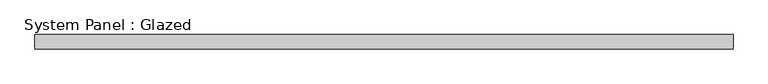
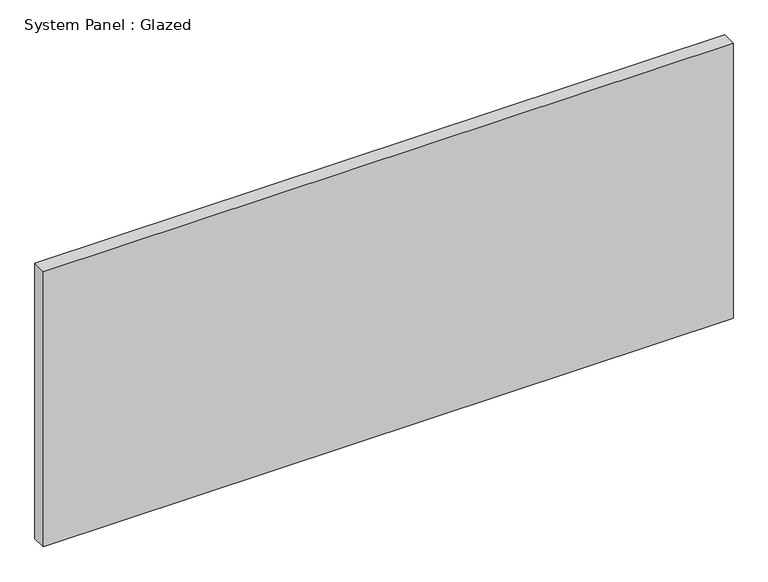
"""IFC4 building model written with IfcOpenShell, lengths in millimetres: plate geometry, System Panel : Glazed."""

from ifc_helpers import new_model, si_unit, origin, origin_with_axes, place, context, project, spatial, polyline, outline, extrude, source, transform, mapped, element, save


def system_panel_glazed_328a0544(model_context):
    return source(origin(), model_context, "Body", "SweptSolid", [
        extrude(outline(polyline([(609.5999999, -44.45), (-609.5999999, -44.45), (-609.5999999, -19.05), (609.5999999, -19.05), (609.5999999, -44.45)])), origin_with_axes(), (0.0, 0.0, 1.0), 514.35),
    ])


if __name__ == "__main__":
    model = new_model("IFC4")
    model_context = context("Model", 3, world=origin())
    ifc_project = project(units=[si_unit("LENGTHUNIT", "METRE", prefix="MILLI")], contexts=[model_context])
    site = spatial("IfcSite", under=ifc_project)
    building = spatial("IfcBuilding", under=site)
    placement = place(None, origin())
    system_panel_glazed_shape = system_panel_glazed_328a0544(model_context)
    element("IfcPlate", 1, ObjectType="System Panel : Glazed", at=placement, inside=building, context=model_context, shape_type="MappedRepresentation", body=[
        mapped(system_panel_glazed_shape, transform((0.0, 0.0, 0.0), x_axis=(1.0, 0.0, 0.0), y_axis=(0.0, 1.0, 0.0), z_axis=(0.0, 0.0, 1.0))),
    ])
    save(model, "model.ifc")

# Revit data of these elements
# Type "System Panel : Glazed"
#   Construction Type Id = "GSP4R"
#   Analytic Construction = "1/8 in Pilkington single glazing"
#   Visual Light Transmittance = 0.9
#   Solar Heat Gain Coefficient = 0.86
#   Heat Transfer Coefficient (U) = 1.18115 BTU/(h·ft²·°F)
#   Define Thermal Properties by = 1
# Element 1 (IfcPlate, "System Panel : Glazed")
#   Materials on its faces: "glass panel 223"
# Materials
#   "glass panel 223": class "Generic", colour RGB 120 120 120, transparency 0, Cost = 0
